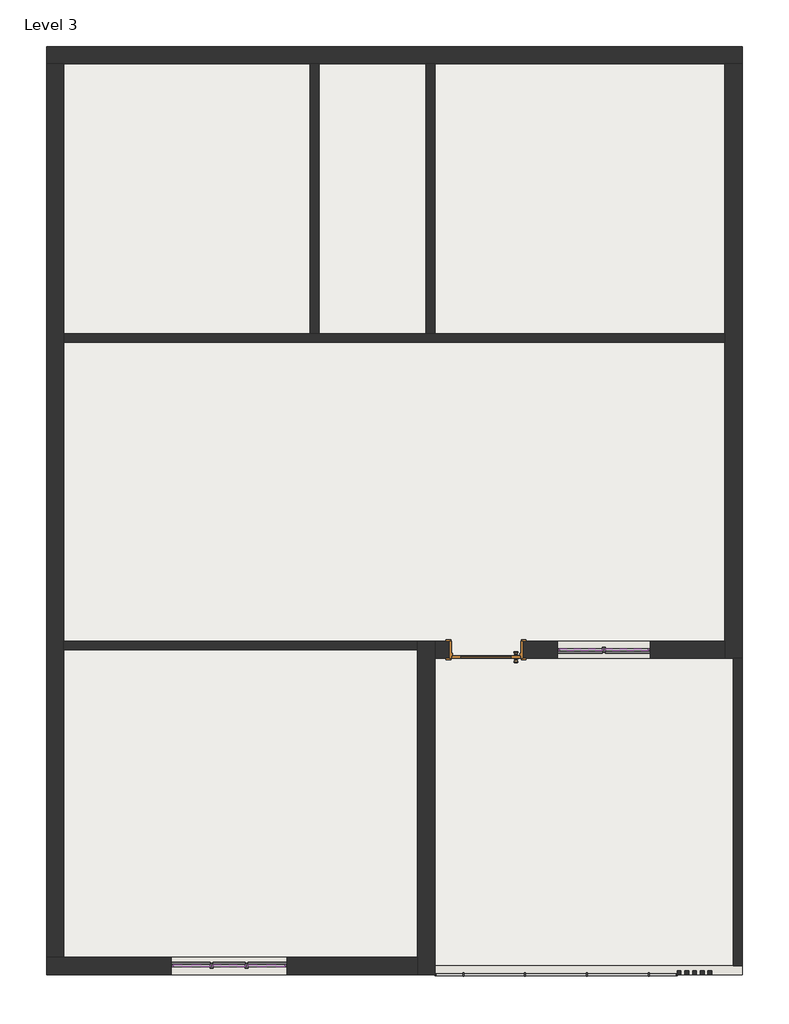
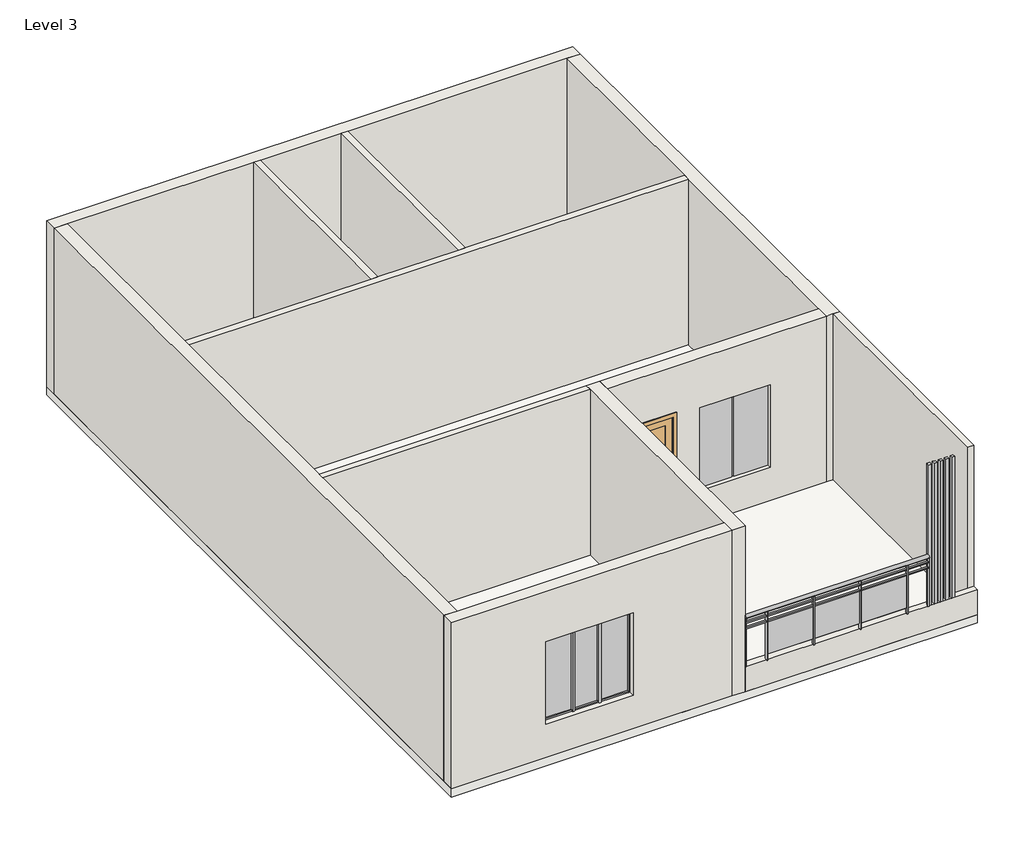
# One storey: 17 members, 12 walls, 5 plates, 1 column, 1 door, 1 railing, 1 slab.
"""IFC4 building model written with IfcOpenShell, lengths in millimetres."""

from ifc_helpers import new_model, si_unit, point, frame, origin, place, context, project, spatial, polyline, ellipse_curve, trimmed, outline, extrude, faceted_brep, transform, mapped, element, save
from ifc_brep_helpers import plane_surface, extruded_surface, advanced_brep
from components import columns_1_columns_1_0c675057, door_3b97b8e7, member_d76f7ec7, member_8b4722c0, member_5dd0e0a2, member_31f2b2ad, member_155beb68, system_panel_glazed_7a35cff4, system_panel_glazed_49ff1c72, system_panel_glazed_817050b2

model = new_model("IFC4")

# Units and contexts
model_context = context("Model", 3, world=origin())
ifc_project = project(units=[si_unit("LENGTHUNIT", "METRE", prefix="MILLI")], contexts=[model_context])

# Site, building, storey
site = spatial("IfcSite", under=ifc_project)
building = spatial("IfcBuilding", under=site)
storey = spatial("IfcBuildingStorey", under=building, Name="Level 3", Elevation=3200.4)

# Column
placement = place(None, origin())
columns_1_columns_1_shape = columns_1_columns_1_0c675057(model_context)
element("IfcColumn", 1, ObjectType="Columns 1 : Columns 1", at=placement, inside=storey, context=model_context, shape_type="MappedRepresentation", body=[
    mapped(columns_1_columns_1_shape, transform((0.0, 0.0, 0.0), x_axis=(1.0, 0.0, 0.0), y_axis=(0.0, 1.0, 0.0), z_axis=(0.0, 0.0, 1.0))),
])

# Door
door_shape = door_3b97b8e7(model_context)
element("IfcDoor", 2, ObjectType="Door-Interior-Single-1_Panel-Wood : 36\" x 84\"", at=placement, inside=storey, context=model_context, shape_type="MappedRepresentation", body=[
    mapped(door_shape, transform((-7775.8551496, 2378.027641, 3200.4), x_axis=(-1.0, 0.0, 0.0), y_axis=(0.0, -1.0, 0.0), z_axis=(0.0, 0.0, 1.0))),
])

# Members
member_shape = member_d76f7ec7(model_context)
element("IfcMember", 3, ObjectType="Rectangular Mullion : 1\" Square", at=placement, inside=storey, context=model_context, shape_type="MappedRepresentation", body=[
    mapped(member_shape, transform((-11916.0551496, -1771.697359, 5334.0), x_axis=(-1.0, 0.0, 0.0), y_axis=(0.0, -1.0, 0.0), z_axis=(0.0, 0.0, 1.0))),
])
element("IfcMember", 4, ObjectType="Rectangular Mullion : 1\" Square", at=placement, inside=storey, context=model_context, shape_type="MappedRepresentation", body=[
    mapped(member_shape, transform((-5616.8551496, 2381.202641, 5334.0), x_axis=(1.0, 0.0, 0.0), y_axis=(0.0, 1.0, 0.0), z_axis=(0.0, 0.0, 1.0))),
])
element("IfcMember", 5, ObjectType="Rectangular Mullion : 1\" Square", at=placement, inside=storey, context=model_context, shape_type="MappedRepresentation", body=[
    mapped(member_shape, transform((-10392.0551496, -1771.697359, 3810.0), x_axis=(1.0, 0.0, 0.0), y_axis=(0.0, -1.0, 0.0), z_axis=(0.0, 0.0, -1.0))),
])
element("IfcMember", 6, ObjectType="Rectangular Mullion : 1\" Square", at=placement, inside=storey, context=model_context, shape_type="MappedRepresentation", body=[
    mapped(member_shape, transform((-6836.0551496, 2381.202641, 3810.0), x_axis=(-1.0, 0.0, 0.0), y_axis=(0.0, 1.0, 0.0), z_axis=(0.0, 0.0, -1.0))),
])
member_2_shape = member_8b4722c0(model_context)
element("IfcMember", 7, ObjectType="Rectangular Mullion : 1\" Square", at=placement, inside=storey, context=model_context, shape_type="MappedRepresentation", body=[
    mapped(member_2_shape, transform((-10417.4551496, -1771.697359, 5334.0), x_axis=(0.0, 0.0, 1.0), y_axis=(0.0, -1.0, 0.0), z_axis=(1.0, 0.0, 0.0))),
])
element("IfcMember", 8, ObjectType="Rectangular Mullion : 1\" Square", at=placement, inside=storey, context=model_context, shape_type="MappedRepresentation", body=[
    mapped(member_2_shape, transform((-11401.7051496, -1771.697359, 5334.0), x_axis=(0.0, 0.0, 1.0), y_axis=(0.0, -1.0, 0.0), z_axis=(1.0, 0.0, 0.0))),
])
element("IfcMember", 9, ObjectType="Rectangular Mullion : 1\" Square", at=placement, inside=storey, context=model_context, shape_type="MappedRepresentation", body=[
    mapped(member_2_shape, transform((-11890.6551496, -1771.697359, 3810.0), x_axis=(0.0, 0.0, -1.0), y_axis=(0.0, -1.0, 0.0), z_axis=(-1.0, 0.0, 0.0))),
])
element("IfcMember", 10, ObjectType="Rectangular Mullion : 1\" Square", at=placement, inside=storey, context=model_context, shape_type="MappedRepresentation", body=[
    mapped(member_2_shape, transform((-10906.4051496, -1771.697359, 3810.0), x_axis=(0.0, 0.0, -1.0), y_axis=(0.0, -1.0, 0.0), z_axis=(-1.0, 0.0, 0.0))),
])
member_3_shape = member_5dd0e0a2(model_context)
element("IfcMember", 11, ObjectType="Rectangular Mullion : 1\" Square", at=placement, inside=storey, context=model_context, shape_type="MappedRepresentation", body=[
    mapped(member_3_shape, transform((-11363.6051496, -1771.697359, 3810.0), x_axis=(0.0, 0.0, -1.0), y_axis=(0.0, -1.0, 0.0), z_axis=(-1.0, 0.0, 0.0))),
])
element("IfcMember", 12, ObjectType="Rectangular Mullion : 1\" Square", at=placement, inside=storey, context=model_context, shape_type="MappedRepresentation", body=[
    mapped(member_3_shape, transform((-10944.5051496, -1771.697359, 5334.0), x_axis=(0.0, 0.0, 1.0), y_axis=(0.0, -1.0, 0.0), z_axis=(1.0, 0.0, 0.0))),
])
member_4_shape = member_31f2b2ad(model_context)
element("IfcMember", 13, ObjectType="Rectangular Mullion : 1\" Square", at=placement, inside=storey, context=model_context, shape_type="MappedRepresentation", body=[
    mapped(member_4_shape, transform((-6810.6551496, 2381.202641, 5334.0), x_axis=(0.0, 0.0, 1.0), y_axis=(0.0, 1.0, 0.0), z_axis=(-1.0, 0.0, 0.0))),
])
element("IfcMember", 14, ObjectType="Rectangular Mullion : 1\" Square", at=placement, inside=storey, context=model_context, shape_type="MappedRepresentation", body=[
    mapped(member_4_shape, transform((-6207.4051496, 2381.202641, 5334.0), x_axis=(0.0, 0.0, 1.0), y_axis=(0.0, 1.0, 0.0), z_axis=(-1.0, 0.0, 0.0))),
])
element("IfcMember", 15, ObjectType="Rectangular Mullion : 1\" Square", at=placement, inside=storey, context=model_context, shape_type="MappedRepresentation", body=[
    mapped(member_4_shape, transform((-5642.2551496, 2381.202641, 3810.0), x_axis=(0.0, 0.0, -1.0), y_axis=(0.0, 1.0, 0.0), z_axis=(1.0, 0.0, 0.0))),
])
element("IfcMember", 16, ObjectType="Rectangular Mullion : 1\" Square", at=placement, inside=storey, context=model_context, shape_type="MappedRepresentation", body=[
    mapped(member_4_shape, transform((-6245.5051496, 2381.202641, 3810.0), x_axis=(0.0, 0.0, -1.0), y_axis=(0.0, 1.0, 0.0), z_axis=(1.0, 0.0, 0.0))),
])
member_5_shape = member_155beb68(model_context)
element("IfcMember", 17, ObjectType="Rectangular Mullion : 1.5\" x 2.5\" rectangular", at=placement, inside=storey, context=model_context, shape_type="MappedRepresentation", body=[
    mapped(member_5_shape, transform((-11382.6551496, -1771.697359, 3810.0), x_axis=(1.0, 0.0, 0.0), y_axis=(0.0, -1.0, 0.0), z_axis=(0.0, 0.0, -1.0))),
])
element("IfcMember", 18, ObjectType="Rectangular Mullion : 1.5\" x 2.5\" rectangular", at=placement, inside=storey, context=model_context, shape_type="MappedRepresentation", body=[
    mapped(member_5_shape, transform((-10925.4551496, -1771.697359, 3810.0), x_axis=(1.0, 0.0, 0.0), y_axis=(0.0, -1.0, 0.0), z_axis=(0.0, 0.0, -1.0))),
])
element("IfcMember", 19, ObjectType="Rectangular Mullion : 1.5\" x 2.5\" rectangular", at=placement, inside=storey, context=model_context, shape_type="MappedRepresentation", body=[
    mapped(member_5_shape, transform((-6226.4551496, 2381.202641, 3810.0), x_axis=(-1.0, 0.0, 0.0), y_axis=(0.0, 1.0, 0.0), z_axis=(0.0, 0.0, -1.0))),
])

# Plates
system_panel_glazed_shape = system_panel_glazed_7a35cff4(model_context)
element("IfcPlate", 20, ObjectType="System Panel : Glazed", at=placement, inside=storey, context=model_context, shape_type="MappedRepresentation", body=[
    mapped(system_panel_glazed_shape, transform((-11658.8801496, -1771.697359, 3810.0), x_axis=(1.0, 0.0, 0.0), y_axis=(0.0, 1.0, 0.0), z_axis=(0.0, 0.0, 1.0))),
])
element("IfcPlate", 21, ObjectType="System Panel : Glazed", at=placement, inside=storey, context=model_context, shape_type="MappedRepresentation", body=[
    mapped(system_panel_glazed_shape, transform((-10649.2301496, -1771.697359, 3810.0), x_axis=(1.0, 0.0, 0.0), y_axis=(0.0, 1.0, 0.0), z_axis=(0.0, 0.0, 1.0))),
])
system_panel_glazed_2_shape = system_panel_glazed_49ff1c72(model_context)
element("IfcPlate", 22, ObjectType="System Panel : Glazed", at=placement, inside=storey, context=model_context, shape_type="MappedRepresentation", body=[
    mapped(system_panel_glazed_2_shape, transform((-11154.0551496, -1771.697359, 3810.0), x_axis=(1.0, 0.0, 0.0), y_axis=(0.0, 1.0, 0.0), z_axis=(0.0, 0.0, 1.0))),
])
system_panel_glazed_3_shape = system_panel_glazed_817050b2(model_context)
element("IfcPlate", 23, ObjectType="System Panel : Glazed", at=placement, inside=storey, context=model_context, shape_type="MappedRepresentation", body=[
    mapped(system_panel_glazed_3_shape, transform((-5912.1301496, 2381.202641, 3810.0), x_axis=(-1.0, 0.0, 0.0), y_axis=(0.0, -1.0, 0.0), z_axis=(0.0, 0.0, 1.0))),
])
element("IfcPlate", 24, ObjectType="System Panel : Glazed", at=placement, inside=storey, context=model_context, shape_type="MappedRepresentation", body=[
    mapped(system_panel_glazed_3_shape, transform((-6540.7801496, 2381.202641, 3810.0), x_axis=(-1.0, 0.0, 0.0), y_axis=(0.0, -1.0, 0.0), z_axis=(0.0, 0.0, 1.0))),
])

# Railing
element("IfcRailing", 25, ObjectType="Glass Panel - Bottom Fill", at=placement, inside=storey, context=model_context, shape_type="SolidModel", body=[
    advanced_brep(
    [(-8448.9551496, -1847.897359, 4572.0), (-8448.9551496, -1924.097359, 4572.0), (-5264.4301496, -1847.897359, 4572.0), (-5264.4301496, -1924.097359, 4572.0)],
    [
        (0, 1, ellipse_curve(frame((-8448.9551496, -1885.997359, 4572.0), z_axis=(-1.0, 0.0, 0.0), x_axis=(0.0, -1.0, 0.0)), 38.1, 28.575)),
        (1, 0, ellipse_curve(frame((-8448.9551496, -1885.997359, 4572.0), z_axis=(-1.0, 0.0, 0.0), x_axis=(0.0, -1.0, 0.0)), 38.1, 28.575)),
        (2, 3, ellipse_curve(frame((-5264.4301496, -1885.997359, 4572.0), z_axis=(1.0, 0.0, 0.0), x_axis=(0.0, -1.0, 0.0)), 38.1, 28.575)),
        (3, 2, ellipse_curve(frame((-5264.4301496, -1885.997359, 4572.0), z_axis=(1.0, 0.0, 0.0), x_axis=(0.0, -1.0, 0.0)), 38.1, 28.575)),
        (0, 2),
        (3, 1),
    ],
    [
        plane_surface(frame((-8448.9551496, -1885.997359, 4572.0), z_axis=(-1.0, 0.0, 0.0), x_axis=(0.0, 1.0, 0.0))),
        plane_surface(frame((-5264.4301496, -1885.997359, 4572.0), z_axis=(1.0, 0.0, 0.0), x_axis=(0.0, 1.0, 0.0))),
        extruded_surface(trimmed(ellipse_curve(frame((-5264.4301496, -1885.997359, 4572.0), z_axis=(-1.0, 0.0, 0.0), x_axis=(0.0, -1.0, 0.0)), 38.1, 28.575), [point((-5264.4301496, -1847.897359, 4572.0))], [point((-5264.4301496, -1924.097359, 4572.0))], True, "CARTESIAN"), (-3184.5250000000005, 0.0, 0.0), 3184.5250000000005),
        extruded_surface(trimmed(ellipse_curve(frame((-5264.4301496, -1885.997359, 4572.0), z_axis=(-1.0, 0.0, 0.0), x_axis=(0.0, -1.0, 0.0)), 38.1, 28.575), [point((-5264.4301496, -1924.097359, 4572.0))], [point((-5264.4301496, -1847.897359, 4572.0))], True, "CARTESIAN"), (-3184.5250000000005, 0.0, 0.0), 3184.5250000000005),
    ],
    [
        (0, [[1, 2]]),
        (1, [[3, 4]]),
        (2, [[-1, 5, -4, 6]]),
        (3, [[-2, -6, -3, -5]]),
    ],
),
    extrude(outline(polyline([(-8448.9551496, -1898.697359), (-8448.9551496, -1873.297359), (-5264.4301496, -1873.297359), (-5264.4301496, -1898.697359), (-8448.9551496, -1898.697359)])), frame((0.0, 0.0, 4457.7), z_axis=(0.0, 0.0, 1.0), x_axis=(1.0, 0.0, 0.0)), (0.0, 0.0, 1.0), 25.4),
    extrude(outline(polyline([(-8448.9551496, -1898.697359), (-8448.9551496, -1873.297359), (-5264.4301496, -1873.297359), (-5264.4301496, -1898.697359), (-8448.9551496, -1898.697359)])), frame((0.0, 0.0, 4356.1), z_axis=(0.0, 0.0, 1.0), x_axis=(1.0, 0.0, 0.0)), (0.0, 0.0, 1.0), 25.4),
    extrude(outline(polyline([(-5643.8426496, -1911.397359), (-5643.8426496, -1860.597359), (-5631.1426496, -1860.597359), (-5631.1426496, -1911.397359), (-5643.8426496, -1911.397359)])), frame((0.0, 0.0, 3657.6), z_axis=(0.0, 0.0, 1.0), x_axis=(1.0, 0.0, 0.0)), (0.0, 0.0, 1.0), 885.825),
    extrude(outline(polyline([(-6450.2926496, -1879.462202), (-5637.4926496, -1879.462202), (-5637.4926496, -1885.812202), (-6450.2926496, -1885.812202), (-6450.2926496, -1879.462202)])), frame((0.0, 0.0, 3759.2), z_axis=(0.0, 0.0, 1.0), x_axis=(1.0, 0.0, 0.0)), (0.0, 0.0, 1.0), 596.9),
    extrude(outline(polyline([(-6456.6426496, -1911.397359), (-6456.6426496, -1860.597359), (-6443.9426496, -1860.597359), (-6443.9426496, -1911.397359), (-6456.6426496, -1911.397359)])), frame((0.0, 0.0, 3657.6), z_axis=(0.0, 0.0, 1.0), x_axis=(1.0, 0.0, 0.0)), (0.0, 0.0, 1.0), 885.825),
    extrude(outline(polyline([(-7263.0926496, -1879.462202), (-6450.2926496, -1879.462202), (-6450.2926496, -1885.812202), (-7263.0926496, -1885.812202), (-7263.0926496, -1879.462202)])), frame((0.0, 0.0, 3759.2), z_axis=(0.0, 0.0, 1.0), x_axis=(1.0, 0.0, 0.0)), (0.0, 0.0, 1.0), 596.9),
    extrude(outline(polyline([(-7269.4426496, -1911.397359), (-7269.4426496, -1860.597359), (-7256.7426496, -1860.597359), (-7256.7426496, -1911.397359), (-7269.4426496, -1911.397359)])), frame((0.0, 0.0, 3657.6), z_axis=(0.0, 0.0, 1.0), x_axis=(1.0, 0.0, 0.0)), (0.0, 0.0, 1.0), 885.825),
    extrude(outline(polyline([(-8075.8926496, -1879.462202), (-7263.0926496, -1879.462202), (-7263.0926496, -1885.812202), (-8075.8926496, -1885.812202), (-8075.8926496, -1879.462202)])), frame((0.0, 0.0, 3759.2), z_axis=(0.0, 0.0, 1.0), x_axis=(1.0, 0.0, 0.0)), (0.0, 0.0, 1.0), 596.9),
    extrude(outline(polyline([(-8082.2426496, -1911.397359), (-8082.2426496, -1860.597359), (-8069.5426496, -1860.597359), (-8069.5426496, -1911.397359), (-8082.2426496, -1911.397359)])), frame((0.0, 0.0, 3657.6), z_axis=(0.0, 0.0, 1.0), x_axis=(1.0, 0.0, 0.0)), (0.0, 0.0, 1.0), 885.825),
    extrude(outline(polyline([(-5277.1301496, -1895.522359), (-5277.1301496, -1876.472359), (-5258.0801496, -1876.472359), (-5258.0801496, -1895.522359), (-5277.1301496, -1895.522359)])), frame((0.0, 0.0, 3657.6), z_axis=(0.0, 0.0, 1.0), x_axis=(1.0, 0.0, 0.0)), (0.0, 0.0, 1.0), 885.825),
    extrude(outline(polyline([(-8455.3051496, -1895.522359), (-8455.3051496, -1876.472359), (-8436.2551496, -1876.472359), (-8436.2551496, -1895.522359), (-8455.3051496, -1895.522359)])), frame((0.0, 0.0, 3657.6), z_axis=(0.0, 0.0, 1.0), x_axis=(1.0, 0.0, 0.0)), (0.0, 0.0, 1.0), 885.825),
])

# Slab
element("IfcSlab", 26, ObjectType="6\" floor", at=placement, inside=storey, context=model_context, shape_type="SweptSolid", body=[
    extrude(outline(polyline([(-4410.3551496, 10306.002641), (-4410.3551496, -1885.997359), (-13554.3551496, -1885.997359), (-13554.3551496, 10306.002641), (-4410.3551496, 10306.002641)])), frame((0.0, 0.0, 3048.0), z_axis=(0.0, 0.0, 1.0), x_axis=(1.0, 0.0, 0.0)), (0.0, 0.0, 1.0), 152.4),
])

# Walls
element("IfcWall", 27, ObjectType="4.5\" INNER WALL", at=placement, inside=storey, context=model_context, shape_type="SweptSolid", body=[
    extrude(outline(polyline([(-13325.7551496, 2495.502641), (-8677.5551496, 2495.502641), (-8677.5551496, 2381.202641), (-13325.7551496, 2381.202641), (-13325.7551496, 2495.502641)])), frame((0.0, 0.0, 3200.4), z_axis=(0.0, 0.0, 1.0), x_axis=(1.0, 0.0, 0.0)), (0.0, 0.0, 1.0), 3048.0),
])
element("IfcWall", 28, ObjectType="4.5\" INNER WALL", at=placement, inside=storey, context=model_context, shape_type="Brep", body=[
    faceted_brep([(-13325.7551496, 6419.802641, 3200.4), (-4638.9551496, 6419.802641, 3200.4), (-4638.9551496, 6419.802641, 6248.4), (-13325.7551496, 6419.802641, 6248.4), (-13325.7551496, 6534.102641, 3200.4), (-13325.7551496, 6534.102641, 6248.4), (-10087.2551496, 6534.102641, 6248.4), (-9972.9551496, 6534.102641, 6248.4), (-8563.2551496, 6534.102641, 6248.4), (-8448.9551496, 6534.102641, 6248.4), (-4638.9551496, 6534.102641, 6248.4), (-4638.9551496, 6534.102641, 3200.4), (-8448.9551496, 6534.102641, 3200.4), (-8563.2551496, 6534.102641, 3200.4), (-9972.9551496, 6534.102641, 3200.4), (-10087.2551496, 6534.102641, 3200.4)], [[[0, 1, 2, 3]], [[4, 5, 6, 7, 8, 9, 10, 11, 12, 13, 14, 15]], [[1, 0, 4, 15, 14, 13, 12, 11]], [[3, 2, 10, 9, 8, 7, 6, 5]], [[2, 1, 11, 10]], [[0, 3, 5, 4]]]),
])
element("IfcWall", 29, ObjectType="4.5\" INNER WALL", at=placement, inside=storey, context=model_context, shape_type="SweptSolid", body=[
    extrude(outline(polyline([(-9972.9551496, 10077.402641), (-9972.9551496, 6534.102641), (-10087.2551496, 6534.102641), (-10087.2551496, 10077.402641), (-9972.9551496, 10077.402641)])), frame((0.0, 0.0, 3200.4), z_axis=(0.0, 0.0, 1.0), x_axis=(1.0, 0.0, 0.0)), (0.0, 0.0, 1.0), 3048.0),
])
element("IfcWall", 30, ObjectType="4.5\" INNER WALL", at=placement, inside=storey, context=model_context, shape_type="SweptSolid", body=[
    extrude(outline(polyline([(-8448.9551496, 10077.402641), (-8448.9551496, 6534.102641), (-8563.2551496, 6534.102641), (-8563.2551496, 10077.402641), (-8448.9551496, 10077.402641)])), frame((0.0, 0.0, 3200.4), z_axis=(0.0, 0.0, 1.0), x_axis=(1.0, 0.0, 0.0)), (0.0, 0.0, 1.0), 3048.0),
])
element("IfcWall", 31, ObjectType="4.5\" INNER WALL", at=placement, inside=storey, context=model_context, shape_type="Brep", body=[
    faceted_brep([(-8448.9551496, -1885.997359, 3200.4), (-4410.3551496, -1885.997359, 3200.4), (-4410.3551496, -1885.997359, 3657.6), (-8448.9551496, -1885.997359, 3657.6), (-8448.9551496, -1771.697359, 3200.4), (-8448.9551496, -1771.697359, 3657.6), (-4410.3551496, -1771.697359, 3657.6), (-4410.3551496, -1771.697359, 3200.4), (-4524.6551496, -1771.697359, 3200.4)], [[[0, 1, 2, 3]], [[4, 5, 6, 7, 8]], [[1, 0, 4, 8, 7]], [[3, 2, 6, 5]], [[0, 3, 5, 4]], [[2, 1, 7, 6]]]),
])
element("IfcWall", 32, ObjectType="4.5\" INNER WALL", at=placement, inside=storey, context=model_context, shape_type="Brep", body=[
    faceted_brep([(-4524.6551496, 2266.902641, 3200.4), (-4524.6551496, -1771.697359, 3200.4), (-4524.6551496, -1771.697359, 6248.4), (-4524.6551496, 2266.902641, 6248.4), (-4410.3551496, 2266.902641, 3200.4), (-4410.3551496, 2266.902641, 6248.4), (-4410.3551496, -1771.697359, 6248.4), (-4410.3551496, -1771.697359, 3657.6), (-4410.3551496, -1771.697359, 3200.4)], [[[0, 1, 2, 3]], [[4, 5, 6, 7, 8]], [[1, 0, 4, 8]], [[3, 2, 6, 5]], [[0, 3, 5, 4]], [[2, 1, 8, 7, 6]]]),
])
element("IfcWall", 33, ObjectType="9\" WALL", at=placement, inside=storey, context=model_context, shape_type="Brep", body=[
    faceted_brep([(-13554.3551496, 10077.402641, 3200.4), (-13325.7551496, 10077.402641, 3200.4), (-10087.2551496, 10077.402641, 3200.4), (-9972.9551496, 10077.402641, 3200.4), (-8563.2551496, 10077.402641, 3200.4), (-8448.9551496, 10077.402641, 3200.4), (-4638.9551496, 10077.402641, 3200.4), (-4410.3551496, 10077.402641, 3200.4), (-4410.3551496, 10077.402641, 6248.4), (-4638.9551496, 10077.402641, 6248.4), (-8448.9551496, 10077.402641, 6248.4), (-8563.2551496, 10077.402641, 6248.4), (-9972.9551496, 10077.402641, 6248.4), (-10087.2551496, 10077.402641, 6248.4), (-13325.7551496, 10077.402641, 6248.4), (-13554.3551496, 10077.402641, 6248.4), (-13554.3551496, 10306.002641, 3200.4), (-13554.3551496, 10306.002641, 6248.4), (-4410.3551496, 10306.002641, 6248.4), (-4410.3551496, 10306.002641, 3200.4)], [[[0, 1, 2, 3, 4, 5, 6, 7, 8, 9, 10, 11, 12, 13, 14, 15]], [[16, 17, 18, 19]], [[7, 6, 5, 4, 3, 2, 1, 0, 16, 19]], [[15, 14, 13, 12, 11, 10, 9, 8, 18, 17]], [[8, 7, 19, 18]], [[0, 15, 17, 16]]]),
])
element("IfcWall", 34, ObjectType="9\" WALL", at=placement, inside=storey, context=model_context, shape_type="Brep", body=[
    faceted_brep([(-4638.9551496, 10077.402641, 3200.4), (-4638.9551496, 6534.102641, 3200.4), (-4638.9551496, 6419.802641, 3200.4), (-4638.9551496, 2495.502641, 3200.4), (-4638.9551496, 2266.902641, 3200.4), (-4638.9551496, 2266.902641, 6248.4), (-4638.9551496, 2495.502641, 6248.4), (-4638.9551496, 6419.802641, 6248.4), (-4638.9551496, 6534.102641, 6248.4), (-4638.9551496, 10077.402641, 6248.4), (-4410.3551496, 10077.402641, 3200.4), (-4410.3551496, 10077.402641, 6248.4), (-4410.3551496, 2266.902641, 6248.4), (-4410.3551496, 2266.902641, 3200.4), (-4524.6551496, 2266.902641, 3200.4), (-4524.6551496, 2266.902641, 6248.4)], [[[0, 1, 2, 3, 4, 5, 6, 7, 8, 9]], [[10, 11, 12, 13]], [[4, 3, 2, 1, 0, 10, 13, 14]], [[9, 8, 7, 6, 5, 15, 12, 11]], [[0, 9, 11, 10]], [[5, 4, 14, 13, 12, 15]]]),
])
element("IfcWall", 35, ObjectType="9\" WALL", at=placement, inside=storey, context=model_context, shape_type="Brep", body=[
    faceted_brep([(-13325.7551496, -1657.397359, 3200.4), (-13325.7551496, 2381.202641, 3200.4), (-13325.7551496, 2495.502641, 3200.4), (-13325.7551496, 6419.802641, 3200.4), (-13325.7551496, 6534.102641, 3200.4), (-13325.7551496, 10077.402641, 3200.4), (-13325.7551496, 10077.402641, 6248.4), (-13325.7551496, 6534.102641, 6248.4), (-13325.7551496, 6419.802641, 6248.4), (-13325.7551496, 2495.502641, 6248.4), (-13325.7551496, 2381.202641, 6248.4), (-13325.7551496, -1657.397359, 6248.4), (-13554.3551496, -1657.397359, 3200.4), (-13554.3551496, -1657.397359, 6248.4), (-13554.3551496, 10077.402641, 6248.4), (-13554.3551496, 10077.402641, 3200.4)], [[[0, 1, 2, 3, 4, 5, 6, 7, 8, 9, 10, 11]], [[12, 13, 14, 15]], [[5, 4, 3, 2, 1, 0, 12, 15]], [[11, 10, 9, 8, 7, 6, 14, 13]], [[0, 11, 13, 12]], [[6, 5, 15, 14]]]),
])
element("IfcWall", 36, ObjectType="9\" WALL", at=placement, inside=storey, context=model_context, shape_type="Brep", body=[
    faceted_brep([(-8448.9551496, -1885.997359, 6248.4), (-8448.9551496, -1885.997359, 3657.6), (-8448.9551496, -1885.997359, 3200.4), (-8448.9551496, -1771.697359, 3200.4), (-8448.9551496, 2266.902641, 3200.4), (-8448.9551496, 2495.502641, 3200.4), (-8448.9551496, 2495.502641, 6248.4), (-8448.9551496, 2266.902641, 6248.4), (-8677.5551496, -1885.997359, 3200.4), (-8677.5551496, -1885.997359, 6248.4), (-8677.5551496, -1657.397359, 6248.4), (-8677.5551496, 2381.202641, 6248.4), (-8677.5551496, 2495.502641, 6248.4), (-8677.5551496, 2495.502641, 3200.4), (-8677.5551496, 2381.202641, 3200.4), (-8677.5551496, -1657.397359, 3200.4)], [[[0, 1, 2, 3, 4, 5, 6, 7]], [[8, 9, 10, 11, 12, 13, 14, 15]], [[5, 4, 3, 2, 8, 15, 14, 13]], [[0, 7, 6, 12, 11, 10, 9]], [[6, 5, 13, 12]], [[0, 9, 8, 2, 1]]]),
])
element("IfcWall", 37, ObjectType="9\" WALL", at=placement, inside=storey, context=model_context, shape_type="SweptSolid", body=[
    extrude(outline(polyline([(6248.4, -4638.9551496), (6248.4, -8448.9551496), (3200.4, -8448.9551496), (3200.4, -8258.4551496), (5359.4, -8258.4551496), (5359.4, -7293.2551496), (3200.4, -7293.2551496), (3200.4, -4638.9551496), (6248.4, -4638.9551496)]), holes=[polyline([(5334.0, -5616.8551496), (3810.0, -5616.8551496), (3810.0, -6836.0551496), (5334.0, -6836.0551496), (5334.0, -5616.8551496)])]), frame((0.0, 2266.902641, 0.0), z_axis=(0.0, 1.0, 0.0), x_axis=(0.0, 0.0, 1.0)), (0.0, 0.0, 1.0), 228.6),
])
element("IfcWall", 38, ObjectType="9\" WALL", at=placement, inside=storey, context=model_context, shape_type="Brep", body=[
    faceted_brep([(-8677.5551496, -1657.397359, 3200.4), (-13325.7551496, -1657.397359, 3200.4), (-13554.3551496, -1657.397359, 3200.4), (-13554.3551496, -1657.397359, 6248.4), (-13325.7551496, -1657.397359, 6248.4), (-8677.5551496, -1657.397359, 6248.4), (-11916.0551496, -1657.397359, 5334.0), (-11916.0551496, -1657.397359, 3810.0), (-10392.0551496, -1657.397359, 3810.0), (-10392.0551496, -1657.397359, 5334.0), (-13554.3551496, -1885.997359, 3200.4), (-8677.5551496, -1885.997359, 3200.4), (-8677.5551496, -1885.997359, 6248.4), (-13554.3551496, -1885.997359, 6248.4), (-11916.0551496, -1885.997359, 3810.0), (-11916.0551496, -1885.997359, 5334.0), (-10392.0551496, -1885.997359, 5334.0), (-10392.0551496, -1885.997359, 3810.0)], [[[0, 1, 2, 3, 4, 5], [6, 7, 8, 9]], [[10, 11, 12, 13], [14, 15, 16, 17]], [[2, 1, 0, 11, 10]], [[5, 4, 3, 13, 12]], [[3, 2, 10, 13]], [[14, 7, 6, 15]], [[15, 6, 9, 16]], [[16, 9, 8, 17]], [[7, 14, 17, 8]], [[5, 12, 11, 0]]]),
])

save(model, "model.ifc")

# Revit data of these elements
# Type "Door-Interior-Single-1_Panel-Wood : 36\" x 84\""
#   Type Mark = "8"
#   Assembly Code = "C1020300"
#   Analytic Construction = "Wooden"
#   Top Rail = 0' - 4 11/16"
#   Thickness = 0' - 1 3/8"
#   Thermal Resistance (R) = 2.5876 (h·ft²·°F)/BTU
#   Swing Angle [instance default] = 90.00°
#   Stiles = 0' - 4 3/4"
#   Rough Width = 3' - 2"
#   Rough Height = 7' - 1"
#   Height = 7' - 0"
#   Width = 3' - 0"
#   Heat Transfer Coefficient (U) = 0.3865 BTU/(h·ft²·°F)
#   Bottom Rail = 0' - 9 1/8"
#   Trim Material = Cherry
#   Panel Material = door
#   Frame Material = door
#   Door Handle Material = Aluminum
#   Visual Light Transmittance = 0
#   Solar Heat Gain Coefficient = 0
#   Wall Closure = (empty or 0)
#   Function = (empty or 0)
# Type "Rectangular Mullion : 1\" Square"
#   built-in parameter 1007304 = 0.0833333 (stored number, unit not read)
#   built-in parameter 1007301 = 0.0416667 (stored number, unit not read)
#   built-in parameter 1007300 = 0.0416667 (stored number, unit not read)
# Type "Rectangular Mullion : 1.5\" x 2.5\" rectangular"
#   built-in parameter 1007304 = 0.208333 (stored number, unit not read)
#   built-in parameter 1007301 = 0.0625 (stored number, unit not read)
#   built-in parameter 1007300 = 0.0625 (stored number, unit not read)
# Type "System Panel : Glazed"
#   Construction Type Id = "GSP4R"
#   Analytic Construction = "1/8 in Pilkington single glazing"
#   Visual Light Transmittance = 0.9
#   Solar Heat Gain Coefficient = 0.86
#   Heat Transfer Coefficient (U) = 1.18115 BTU/(h·ft²·°F)
#   Define Thermal Properties by = 1
# Type "Glass Panel - Bottom Fill"
#   Assembly Code = "C2010400"
#   built-in parameter 1008612 = 0.0416667 (stored number, unit not read)
#   built-in parameter 1008611 = 0.0416667 (stored number, unit not read)
#   built-in parameter 1008609 = 0.333333 (stored number, unit not read)
#   built-in parameter 1008604 = 0.166667 (stored number, unit not read)
#   built-in parameter 1008603 = 0.166667 (stored number, unit not read)
#   Railing Height = 3' - 0"
#   built-in parameter 1008630 = 2
#   built-in parameter 1008610 = 2
#   built-in parameter 1008618 = Baluster - Square : 3/4"
# Type "6\" floor"
#   Assembly Code = "B1010"
#   Function = 0
#   Layers, outside or top first: 0' - 6" no material (function 1)
# Type "4.5\" INNER WALL"
#   Assembly Code = "B2010"
#   Layers, outside or top first: 0' - 4 1/2" "Damp-proofing" (function 1)
# Type "9\" WALL"
#   Assembly Code = "B2010"
#   Layers, outside or top first: 0' - 9" "Analytical Surface - Exterior Walls" (function 1)
# Element 1 (IfcColumn, "Columns 1 : Columns 1")
#   Phase Created = New Construction
#   Materials on its faces: "Damp-proofing"
# Element 2 (IfcDoor, "Door-Interior-Single-1_Panel-Wood : 36\" x 84\"")
#   Swing Angle = 90.00°
#   Phase Created = New Construction
#   Materials on its faces: "Aluminum", "door", "Cherry"
# Elements 3, 4, 5, 6, 7, 8, 9, 10, 11, 12, 13, 14, 15, 16 (IfcMember, "Rectangular Mullion : 1\" Square")
#   Phase Created = New Construction
# Elements 17, 18, 19 (IfcMember, "Rectangular Mullion : 1.5\" x 2.5\" rectangular")
#   Phase Created = New Construction
#   Materials on its faces: "mullions"
# Elements 20, 21, 22, 23, 24 (IfcPlate, "System Panel : Glazed")
#   Phase Created = New Construction
#   Materials on its faces: "Glass"
# Element 25 (IfcRailing, "Glass Panel - Bottom Fill")
#   built-in parameter 1008621 = 1.5 (stored number, unit not read)
#   Phase Created = New Construction
#   Materials on its faces: "Glass"
# Element 26 (IfcSlab, "6\" floor")
#   Height Offset From Level = 0' - 0"
#   Phase Created = New Construction
#   Materials on its faces: "Default Floor"
# Elements 27, 28, 29, 30, 32 (IfcWall, "4.5\" INNER WALL")
#   Top Offset = 0' - 0"
#   Base Offset = 0' - 0"
#   wall height = 10' - 0"
#   Phase Created = New Construction
#   Base Constraint = Level 3
#   Top Constraint = Level 4
#   Materials on its faces: "Damp-proofing"
# Element 31 (IfcWall, "4.5\" INNER WALL")
#   Top Offset = 0' - 0"
#   Base Offset = 0' - 0"
#   Unconnected Height = 1' - 6"
#   wall height = 1' - 6"
#   Phase Created = New Construction
#   Base Constraint = Level 3
#   Materials on its faces: "Damp-proofing"
# Elements 33, 34, 35, 36, 37, 38 (IfcWall, "9\" WALL")
#   Top Offset = 0' - 0"
#   Base Offset = 0' - 0"
#   wall height = 10' - 0"
#   Phase Created = New Construction
#   Base Constraint = Level 3
#   Top Constraint = Level 4
#   Materials on its faces: "Analytical Surface - Exterior Walls"
# Materials
#   "Cherry": class "Wood", colour RGB 226 177 128, transparency 0, Description = "Prunus Serotina", Cost = 0
#   "door": class "Generic", colour RGB 120 120 120, transparency 0, Cost = 0
#   "Aluminum": class "Metal", colour RGB 247 247 247, transparency 0, Description = "Aluminum 6061", Cost = 0
#   "Damp-proofing": class "Generic", colour RGB 127 127 127, transparency 0, Description = "Damp-proofing", Cost = 0
#   "Analytical Surface - Exterior Walls": colour RGB 133 178 44, transparency 0.5, Cost = 0
#   "mullions": class "Generic", colour RGB 120 120 120, transparency 0, Cost = 0
#   "Glass": class "Glass", colour RGB 0 128 192, transparency 0.75, Description = "Soda Lime Glass", Cost = 0
#   "Default Floor": colour RGB 128 128 128, transparency 0, Cost = 0
